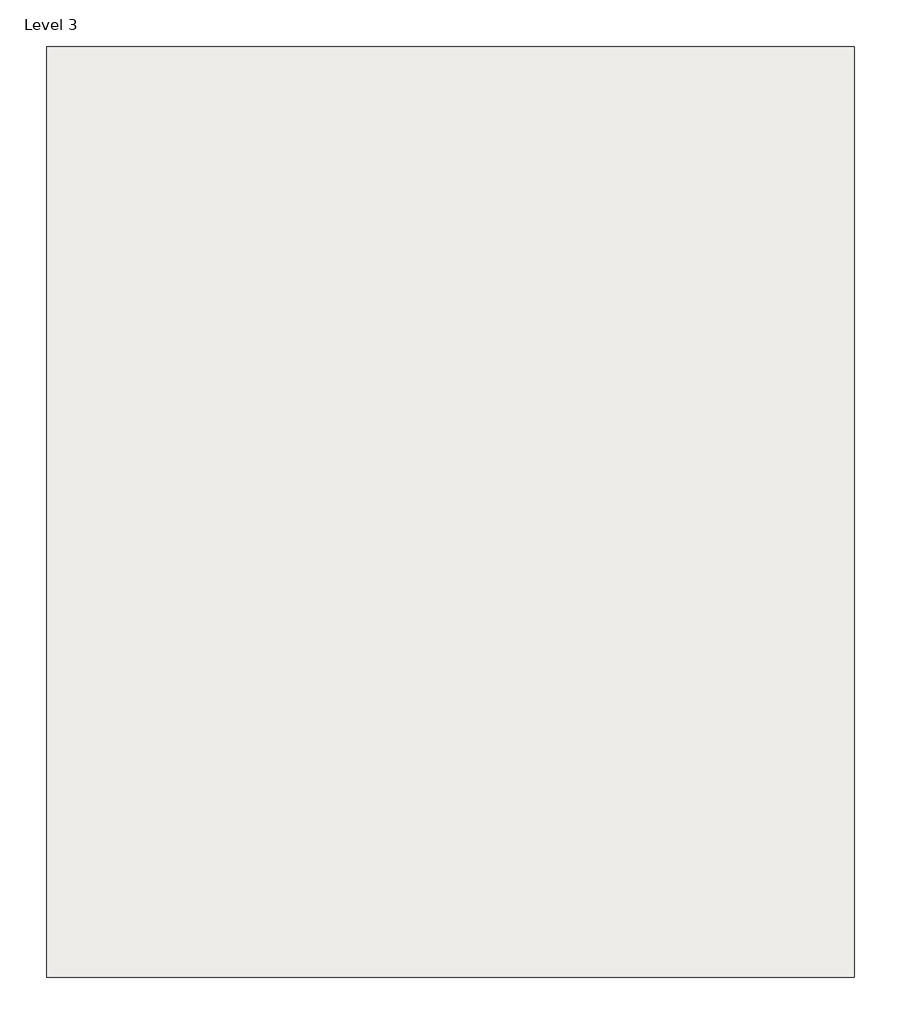
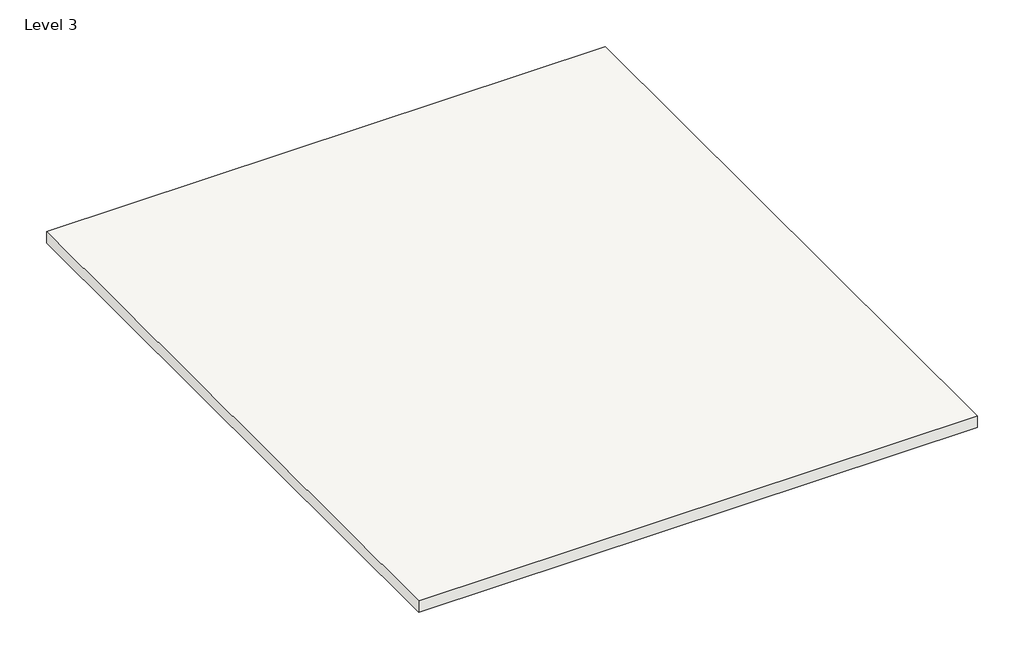
# One storey: 1 roof.
"""IFC4 building model written with IfcOpenShell, lengths in millimetres."""

from ifc_helpers import new_model, si_unit, frame, origin, place, context, project, spatial, polyline, outline, extrude, element, save

model = new_model("IFC4")

# Units and contexts
model_context = context("Model", 3, world=origin())
ifc_project = project(units=[si_unit("LENGTHUNIT", "METRE", prefix="MILLI")], contexts=[model_context])

# Site, building, storey
site = spatial("IfcSite", under=ifc_project)
building = spatial("IfcBuilding", under=site)
storey = spatial("IfcBuildingStorey", under=building, Name="Level 3", Elevation=6096.0)

# Roof
placement = place(None, origin())
element("IfcRoof", 1, ObjectType="Generic - 12\"", at=placement, inside=storey, context=model_context, shape_type="SweptSolid", body=[
    extrude(outline(polyline([(-17929.0047537, -5297.5428796), (-4213.0047537, -5297.5428796), (-4213.0047537, -21109.0428796), (-17929.0047537, -21109.0428796), (-17929.0047537, -5297.5428796)])), frame((0.0, 0.0, 6096.0), z_axis=(0.0, 0.0, 1.0), x_axis=(1.0, 0.0, 0.0)), (0.0, 0.0, 1.0), 304.8),
])

save(model, "model.ifc")

# Revit data of these elements
# Type "Generic - 12\""
#   Assembly Code = "B1020"
#   Layers, outside or top first: 1' - 0" no material (function 1)
# Element 1 (IfcRoof, "Generic - 12\"")
#   built-in parameter 1001705 = 21 (stored number, unit not read)
#   built-in parameter 1001710 = 33615
#   Phase Created = New Construction
#   Materials on its faces: "Default Roof"
# Materials
#   "Default Roof": colour RGB 88 101 114, transparency 0, Cost = 0
